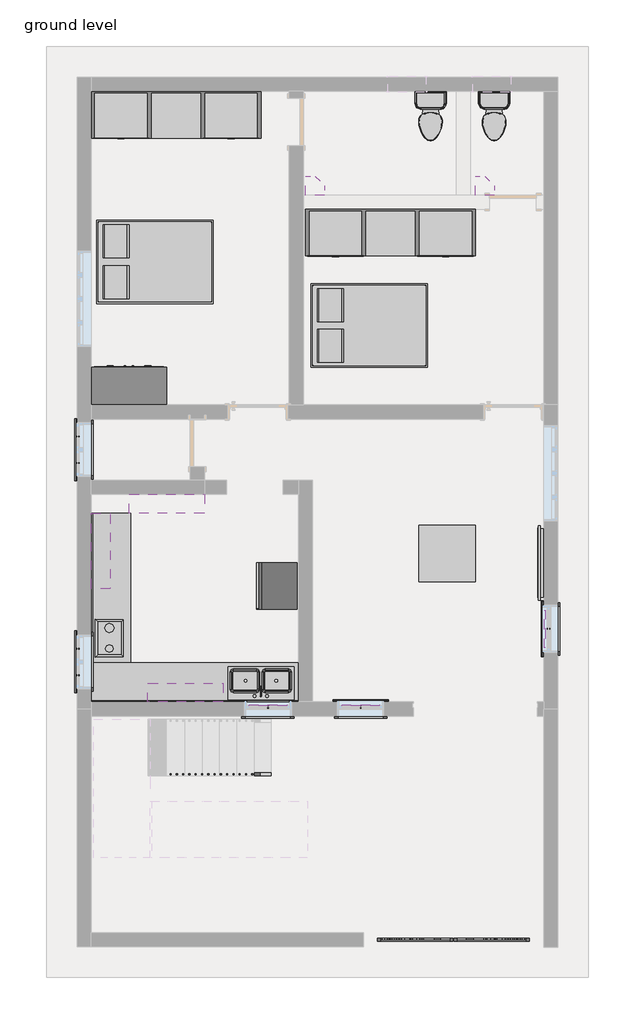
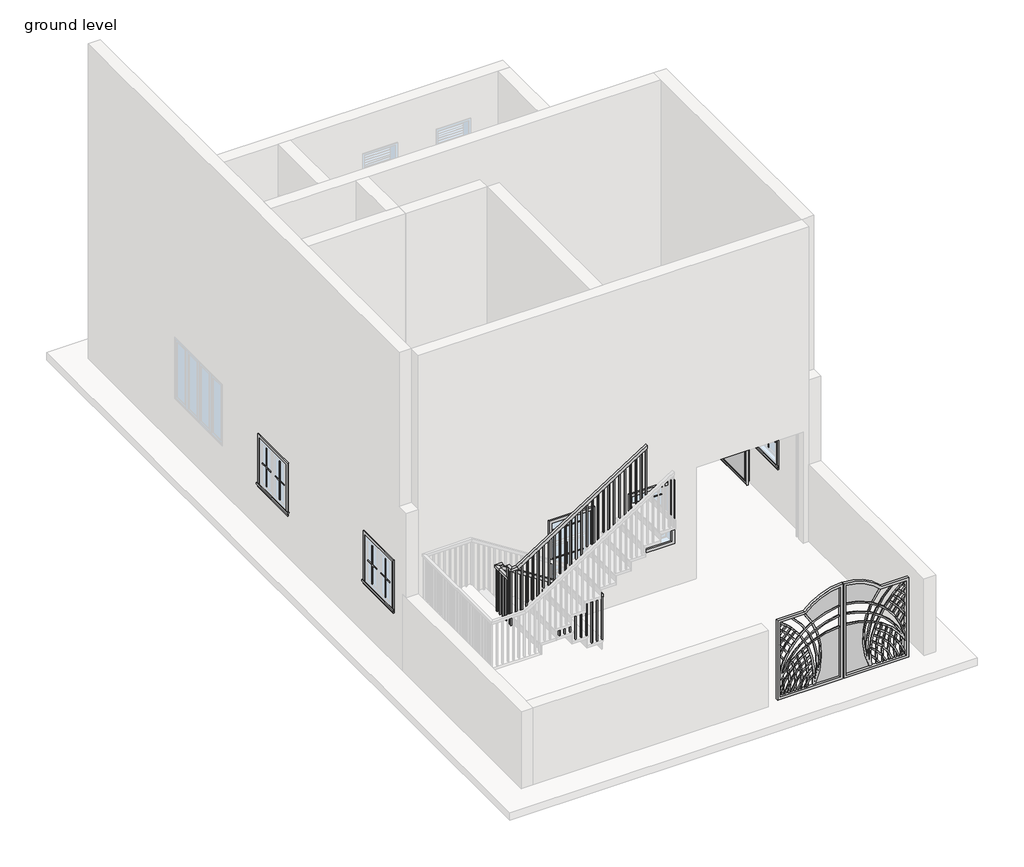
# One storey, part 3 of 3: 23 proxies, 16 furniture elements, 5 flow terminals, 1 railing.
"""IFC4 building model written with IfcOpenShell, lengths in millimetres."""

from ifc_helpers import new_model, si_unit, frame, origin, place, context, project, spatial, polyline, outline, extrude, faceted_brep, transform, mapped, element, save
from components import generic_models_6bc30956, proxy_3c1fa1d0, muntin_pattern_2x2_muntin_pattern_2x2_b3fe6957, muntin_pattern_2x2_muntin_pattern_2x2_3e0ecaf2, muntin_pattern_2x2_muntin_pattern_2x2_b8ba09c9, proxy_76352e5b, trim_window_exterior_flat_with_sill_41619996, trim_window_exterior_flat_with_sill_6cd3ad68, trim_window_interior_flat_picture_frame_51c85655, trim_window_interior_flat_picture_frame_840a62db, flow_terminal_080557f2, flow_terminal_a53be723, toilet_domestic_3d_toilet_domestic_3d_ba6479b0, toilet_domestic_3d_toilet_domestic_3d_30431060, furniture_9b4ba0d7, furniture_3428e43d, furniture_97fe820d, furniture_b58f7881, furniture_05b7e736, furniture_e3ff1115, furniture_1f19b6cd, furniture_8a11f05f, furniture_5e39d705, furniture_f491f192, furniture_82e269c4

model = new_model("IFC4")

# Units and contexts
model_context = context("Model", 3, world=origin())
ifc_project = project(units=[si_unit("LENGTHUNIT", "METRE", prefix="MILLI")], contexts=[model_context])

# Site, building, storey
site = spatial("IfcSite", under=ifc_project)
building = spatial("IfcBuilding", under=site)
storey = spatial("IfcBuildingStorey", under=building, Name="ground level", Elevation=609.6)

# Proxies
placement = place(None, origin())
generic_models_shape = generic_models_6bc30956(model_context)
element("IfcBuildingElementProxy", 1, Name="Generic Models", at=placement, inside=storey, context=model_context, shape_type="MappedRepresentation", body=[
    mapped(generic_models_shape, transform((34462.4566163, 5742.2730552, 609.6), x_axis=(1.0, 0.0, 0.0), y_axis=(0.0, 1.0, 0.0), z_axis=(0.0, 0.0, 1.0))),
])
proxy_shape = proxy_3c1fa1d0(model_context)
element("IfcBuildingElementProxy", 2, Name="Cook Top-2 Unit : 12\" x 18\" 2", ObjectType="Cook Top-2 Unit : 12\" x 18\" 2", at=placement, inside=storey, context=model_context, shape_type="MappedRepresentation", body=[
    mapped(proxy_shape, transform((28826.8316163, 10560.2732596, 609.6), x_axis=(1.0, 0.0, 0.0), y_axis=(0.0, 1.0, 0.0), z_axis=(0.0, 0.0, 1.0))),
])
muntin_pattern_2x2_muntin_pattern_2x2_shape = muntin_pattern_2x2_muntin_pattern_2x2_b3fe6957(model_context)
element("IfcBuildingElementProxy", 3, Name="Muntin Pattern_2x2 : Muntin Pattern_2x2", ObjectType="Muntin Pattern_2x2 : Muntin Pattern_2x2", at=placement, inside=storey, context=model_context, shape_type="MappedRepresentation", body=[
    mapped(muntin_pattern_2x2_muntin_pattern_2x2_shape, transform((28391.8566163, 13424.1855552, 1593.85), x_axis=(0.0, 1.0, 0.0), y_axis=(-1.0, 0.0, 0.0), z_axis=(0.0, 0.0, 1.0))),
])
element("IfcBuildingElementProxy", 4, Name="Muntin Pattern_2x2 : Muntin Pattern_2x2", ObjectType="Muntin Pattern_2x2 : Muntin Pattern_2x2", at=placement, inside=storey, context=model_context, shape_type="MappedRepresentation", body=[
    mapped(muntin_pattern_2x2_muntin_pattern_2x2_shape, transform((28391.8566163, 9995.1855552, 1746.25), x_axis=(0.0, 1.0, 0.0), y_axis=(-1.0, 0.0, 0.0), z_axis=(0.0, 0.0, 1.0))),
])
muntin_pattern_2x2_muntin_pattern_2x2_2_shape = muntin_pattern_2x2_muntin_pattern_2x2_3e0ecaf2(model_context)
element("IfcBuildingElementProxy", 5, Name="Muntin Pattern_2x2 : Muntin Pattern_2x2", ObjectType="Muntin Pattern_2x2 : Muntin Pattern_2x2", at=placement, inside=storey, context=model_context, shape_type="MappedRepresentation", body=[
    mapped(muntin_pattern_2x2_muntin_pattern_2x2_2_shape, transform((28391.8566163, 13852.8105552, 1593.85), x_axis=(0.0, -1.0, 0.0), y_axis=(1.0, 0.0, 0.0), z_axis=(0.0, 0.0, 1.0))),
])
element("IfcBuildingElementProxy", 6, Name="Muntin Pattern_2x2 : Muntin Pattern_2x2", ObjectType="Muntin Pattern_2x2 : Muntin Pattern_2x2", at=placement, inside=storey, context=model_context, shape_type="MappedRepresentation", body=[
    mapped(muntin_pattern_2x2_muntin_pattern_2x2_2_shape, transform((28391.8566163, 10423.8105552, 1746.25), x_axis=(0.0, -1.0, 0.0), y_axis=(1.0, 0.0, 0.0), z_axis=(0.0, 0.0, 1.0))),
])
muntin_pattern_2x2_muntin_pattern_2x2_3_shape = muntin_pattern_2x2_muntin_pattern_2x2_b8ba09c9(model_context)
element("IfcBuildingElementProxy", 7, Name="Muntin Pattern_2x2 : Muntin Pattern_2x2", ObjectType="Muntin Pattern_2x2 : Muntin Pattern_2x2", at=placement, inside=storey, context=model_context, shape_type="MappedRepresentation", body=[
    mapped(muntin_pattern_2x2_muntin_pattern_2x2_3_shape, transform((32967.0316163, 9526.8730552, 2130.425), x_axis=(1.0, 0.0, 0.0), y_axis=(0.0, 1.0, 0.0), z_axis=(0.0, 0.0, 1.0))),
])
element("IfcBuildingElementProxy", 8, Name="Muntin Pattern_2x2 : Muntin Pattern_2x2", ObjectType="Muntin Pattern_2x2 : Muntin Pattern_2x2", at=placement, inside=storey, context=model_context, shape_type="MappedRepresentation", body=[
    mapped(muntin_pattern_2x2_muntin_pattern_2x2_3_shape, transform((32967.0316163, 9482.4230552, 1600.2), x_axis=(1.0, 0.0, 0.0), y_axis=(0.0, 1.0, 0.0), z_axis=(0.0, 0.0, 1.0))),
])
element("IfcBuildingElementProxy", 9, Name="Muntin Pattern_2x2 : Muntin Pattern_2x2", ObjectType="Muntin Pattern_2x2 : Muntin Pattern_2x2", at=placement, inside=storey, context=model_context, shape_type="MappedRepresentation", body=[
    mapped(muntin_pattern_2x2_muntin_pattern_2x2_3_shape, transform((35961.0566163, 10742.8980552, 2130.425), x_axis=(0.0, 1.0, 0.0), y_axis=(-1.0, 0.0, 0.0), z_axis=(0.0, 0.0, 1.0))),
])
element("IfcBuildingElementProxy", 10, Name="Muntin Pattern_2x2 : Muntin Pattern_2x2", ObjectType="Muntin Pattern_2x2 : Muntin Pattern_2x2", at=placement, inside=storey, context=model_context, shape_type="MappedRepresentation", body=[
    mapped(muntin_pattern_2x2_muntin_pattern_2x2_3_shape, transform((36005.5066163, 10742.8980552, 1600.2), x_axis=(0.0, 1.0, 0.0), y_axis=(-1.0, 0.0, 0.0), z_axis=(0.0, 0.0, 1.0))),
])
element("IfcBuildingElementProxy", 11, Name="Muntin Pattern_2x2 : Muntin Pattern_2x2", ObjectType="Muntin Pattern_2x2 : Muntin Pattern_2x2", at=placement, inside=storey, context=model_context, shape_type="MappedRepresentation", body=[
    mapped(muntin_pattern_2x2_muntin_pattern_2x2_3_shape, transform((31468.4316163, 9526.8730552, 2130.425), x_axis=(1.0, 0.0, 0.0), y_axis=(0.0, 1.0, 0.0), z_axis=(0.0, 0.0, 1.0))),
])
element("IfcBuildingElementProxy", 12, Name="Muntin Pattern_2x2 : Muntin Pattern_2x2", ObjectType="Muntin Pattern_2x2 : Muntin Pattern_2x2", at=placement, inside=storey, context=model_context, shape_type="MappedRepresentation", body=[
    mapped(muntin_pattern_2x2_muntin_pattern_2x2_3_shape, transform((31468.4316163, 9482.4230552, 1600.2), x_axis=(1.0, 0.0, 0.0), y_axis=(0.0, 1.0, 0.0), z_axis=(0.0, 0.0, 1.0))),
])
proxy_2_shape = proxy_76352e5b(model_context)
element("IfcBuildingElementProxy", 13, Name="Refrigerator-Built-in : 30\" x 24\" LH", ObjectType="Refrigerator-Built-in : 30\" x 24\" LH", at=placement, inside=storey, context=model_context, shape_type="MappedRepresentation", body=[
    mapped(proxy_2_shape, transform((31644.2555878, 11435.0480552, 609.6), x_axis=(0.0, 1.0, 0.0), y_axis=(-1.0, 0.0, 0.0), z_axis=(0.0, 0.0, 1.0))),
])
trim_window_exterior_flat_with_sill_shape = trim_window_exterior_flat_with_sill_41619996(model_context)
element("IfcBuildingElementProxy", 14, Name="Trim-Window-Exterior-Flat : with Sill", ObjectType="Trim-Window-Exterior-Flat : with Sill", at=placement, inside=storey, context=model_context, shape_type="MappedRepresentation", body=[
    mapped(trim_window_exterior_flat_with_sill_shape, transform((28382.3316163, 13638.4980552, 2438.4), x_axis=(0.0, -1.0, 0.0), y_axis=(0.0, 0.0, 1.0), z_axis=(-1.0, 0.0, 0.0))),
])
element("IfcBuildingElementProxy", 15, Name="Trim-Window-Exterior-Flat : with Sill", ObjectType="Trim-Window-Exterior-Flat : with Sill", at=placement, inside=storey, context=model_context, shape_type="MappedRepresentation", body=[
    mapped(trim_window_exterior_flat_with_sill_shape, transform((28382.3316163, 10209.4980552, 2590.8), x_axis=(0.0, -1.0, 0.0), y_axis=(0.0, 0.0, 1.0), z_axis=(-1.0, 0.0, 0.0))),
])
trim_window_exterior_flat_with_sill_2_shape = trim_window_exterior_flat_with_sill_6cd3ad68(model_context)
element("IfcBuildingElementProxy", 16, Name="Trim-Window-Exterior-Flat : with Sill", ObjectType="Trim-Window-Exterior-Flat : with Sill", at=placement, inside=storey, context=model_context, shape_type="MappedRepresentation", body=[
    mapped(trim_window_exterior_flat_with_sill_2_shape, transform((32967.0316163, 9561.7980552, 2692.4), x_axis=(-1.0, 0.0, 0.0), y_axis=(0.0, 0.0, 1.0), z_axis=(0.0, 1.0, 0.0))),
])
element("IfcBuildingElementProxy", 17, Name="Trim-Window-Exterior-Flat : with Sill", ObjectType="Trim-Window-Exterior-Flat : with Sill", at=placement, inside=storey, context=model_context, shape_type="MappedRepresentation", body=[
    mapped(trim_window_exterior_flat_with_sill_2_shape, transform((35926.1316163, 10742.8980552, 2692.4), x_axis=(0.0, -1.0, 0.0), y_axis=(0.0, 0.0, 1.0), z_axis=(-1.0, 0.0, 0.0))),
])
element("IfcBuildingElementProxy", 18, Name="Trim-Window-Exterior-Flat : with Sill", ObjectType="Trim-Window-Exterior-Flat : with Sill", at=placement, inside=storey, context=model_context, shape_type="MappedRepresentation", body=[
    mapped(trim_window_exterior_flat_with_sill_2_shape, transform((31468.4316163, 9561.7980552, 2692.4), x_axis=(-1.0, 0.0, 0.0), y_axis=(0.0, 0.0, 1.0), z_axis=(0.0, 1.0, 0.0))),
])
trim_window_interior_flat_picture_frame_shape = trim_window_interior_flat_picture_frame_51c85655(model_context)
element("IfcBuildingElementProxy", 19, Name="Trim-Window-Interior-Flat : Picture Frame", ObjectType="Trim-Window-Interior-Flat : Picture Frame", at=placement, inside=storey, context=model_context, shape_type="MappedRepresentation", body=[
    mapped(trim_window_interior_flat_picture_frame_shape, transform((28610.9316163, 13638.4980552, 2438.4), x_axis=(0.0, 1.0, 0.0), y_axis=(0.0, 0.0, 1.0), z_axis=(1.0, 0.0, 0.0))),
])
element("IfcBuildingElementProxy", 20, Name="Trim-Window-Interior-Flat : Picture Frame", ObjectType="Trim-Window-Interior-Flat : Picture Frame", at=placement, inside=storey, context=model_context, shape_type="MappedRepresentation", body=[
    mapped(trim_window_interior_flat_picture_frame_shape, transform((28610.9316163, 10209.4980552, 2590.8), x_axis=(0.0, 1.0, 0.0), y_axis=(0.0, 0.0, 1.0), z_axis=(1.0, 0.0, 0.0))),
])
trim_window_interior_flat_picture_frame_2_shape = trim_window_interior_flat_picture_frame_840a62db(model_context)
element("IfcBuildingElementProxy", 21, Name="Trim-Window-Interior-Flat : Picture Frame", ObjectType="Trim-Window-Interior-Flat : Picture Frame", at=placement, inside=storey, context=model_context, shape_type="MappedRepresentation", body=[
    mapped(trim_window_interior_flat_picture_frame_2_shape, transform((32967.0316163, 9333.1980552, 2692.4), x_axis=(1.0, 0.0, 0.0), y_axis=(0.0, 0.0, 1.0), z_axis=(0.0, -1.0, 0.0))),
])
element("IfcBuildingElementProxy", 22, Name="Trim-Window-Interior-Flat : Picture Frame", ObjectType="Trim-Window-Interior-Flat : Picture Frame", at=placement, inside=storey, context=model_context, shape_type="MappedRepresentation", body=[
    mapped(trim_window_interior_flat_picture_frame_2_shape, transform((36154.7316163, 10742.8980552, 2692.4), x_axis=(0.0, 1.0, 0.0), y_axis=(0.0, 0.0, 1.0), z_axis=(1.0, 0.0, 0.0))),
])
element("IfcBuildingElementProxy", 23, Name="Trim-Window-Interior-Flat : Picture Frame", ObjectType="Trim-Window-Interior-Flat : Picture Frame", at=placement, inside=storey, context=model_context, shape_type="MappedRepresentation", body=[
    mapped(trim_window_interior_flat_picture_frame_2_shape, transform((31468.4316163, 9333.1980552, 2692.4), x_axis=(1.0, 0.0, 0.0), y_axis=(0.0, 0.0, 1.0), z_axis=(0.0, -1.0, 0.0))),
])

# Flow terminals
flow_terminal_shape = flow_terminal_080557f2(model_context)
element("IfcFlowTerminal", 24, ObjectType="Sink - Mop : 28\"x28\" 2", at=placement, inside=storey, context=model_context, shape_type="MappedRepresentation", body=[
    mapped(flow_terminal_shape, transform((32078.0316163, 17753.2980552, 1828.8), x_axis=(0.0, 1.0, 0.0), y_axis=(-1.0, 0.0, 0.0), z_axis=(0.0, 0.0, 1.0))),
])
element("IfcFlowTerminal", 25, ObjectType="Sink - Mop : 28\"x28\" 2", at=placement, inside=storey, context=model_context, shape_type="MappedRepresentation", body=[
    mapped(flow_terminal_shape, transform((34821.2316163, 17753.2980552, 1828.8), x_axis=(0.0, 1.0, 0.0), y_axis=(-1.0, 0.0, 0.0), z_axis=(0.0, 0.0, 1.0))),
])
flow_terminal_2_shape = flow_terminal_a53be723(model_context)
element("IfcFlowTerminal", 26, ObjectType="Sink Kitchen-Double : 42\" x 21\"", at=placement, inside=storey, context=model_context, shape_type="MappedRepresentation", body=[
    mapped(flow_terminal_2_shape, transform((31369.8208569, 9868.9434563, 609.6), x_axis=(-1.0, 0.0, 0.0), y_axis=(0.0, -1.0, 0.0), z_axis=(0.0, 0.0, 1.0))),
])
toilet_domestic_3d_toilet_domestic_3d_shape = toilet_domestic_3d_toilet_domestic_3d_ba6479b0(model_context)
toilet_domestic_3d_toilet_domestic_3d_2_shape = toilet_domestic_3d_toilet_domestic_3d_30431060(model_context)
element("IfcFlowTerminal", 27, ObjectType="Toilet-Domestic-3D : Toilet-Domestic-3D", at=placement, inside=storey, context=model_context, shape_type="MappedRepresentation", body=[
    mapped(toilet_domestic_3d_toilet_domestic_3d_shape, transform((34097.3316163, 18935.0020278, 609.6), x_axis=(1.0, 0.0, 0.0), y_axis=(0.0, 1.0, 0.0), z_axis=(0.0, 0.0, 1.0))),
    mapped(toilet_domestic_3d_toilet_domestic_3d_2_shape, transform((34097.3316163, 18935.0020278, 609.6), x_axis=(1.0, 0.0, 0.0), y_axis=(0.0, 1.0, 0.0), z_axis=(0.0, 0.0, 1.0))),
])
element("IfcFlowTerminal", 28, ObjectType="Toilet-Domestic-3D : Toilet-Domestic-3D", at=placement, inside=storey, context=model_context, shape_type="MappedRepresentation", body=[
    mapped(toilet_domestic_3d_toilet_domestic_3d_shape, transform((35126.0316163, 18935.0020278, 609.6), x_axis=(1.0, 0.0, 0.0), y_axis=(0.0, 1.0, 0.0), z_axis=(0.0, 0.0, 1.0))),
    mapped(toilet_domestic_3d_toilet_domestic_3d_2_shape, transform((35126.0316163, 18935.0020278, 609.6), x_axis=(1.0, 0.0, 0.0), y_axis=(0.0, 1.0, 0.0), z_axis=(0.0, 0.0, 1.0))),
])

# Furniture
furniture_shape = furniture_9b4ba0d7(model_context)
element("IfcFurniture", 29, ObjectType="36\"", at=placement, inside=storey, context=model_context, shape_type="MappedRepresentation", body=[
    mapped(furniture_shape, transform((28610.9316163, 12133.8603503, 609.6), x_axis=(0.0, 1.0, 0.0), y_axis=(-1.0, 0.0, 0.0), z_axis=(0.0, 0.0, 1.0))),
])
furniture_2_shape = furniture_3428e43d(model_context)
element("IfcFurniture", 30, ObjectType="48\"", at=placement, inside=storey, context=model_context, shape_type="MappedRepresentation", body=[
    mapped(furniture_2_shape, transform((30225.7765763, 9561.7980552, 609.6), x_axis=(-1.0, 0.0, 0.0), y_axis=(0.0, -1.0, 0.0), z_axis=(0.0, 0.0, 1.0))),
])
element("IfcFurniture", 31, ObjectType="48\"", at=placement, inside=storey, context=model_context, shape_type="MappedRepresentation", body=[
    mapped(furniture_2_shape, transform((28610.9316163, 10994.9530952, 609.6), x_axis=(0.0, 1.0, 0.0), y_axis=(-1.0, 0.0, 0.0), z_axis=(0.0, 0.0, 1.0))),
])
furniture_3_shape = furniture_97fe820d(model_context)
element("IfcFurniture", 32, ObjectType="Base Cabinet-Corner Unit-Square : 36\"", at=placement, inside=storey, context=model_context, shape_type="MappedRepresentation", body=[
    mapped(furniture_3_shape, transform((29137.6693213, 9561.7980552, 609.6), x_axis=(-1.0, 0.0, 0.0), y_axis=(0.0, -1.0, 0.0), z_axis=(0.0, 0.0, 1.0))),
])
furniture_4_shape = furniture_b58f7881(model_context)
element("IfcFurniture", 33, ObjectType="Bed-Box : Double 53\" x 74\"", at=placement, inside=storey, context=model_context, shape_type="MappedRepresentation", body=[
    mapped(furniture_4_shape, transform((29405.2021081, 16334.6455962, 609.6), x_axis=(0.0, 1.0, 0.0), y_axis=(-1.0, 0.0, 0.0), z_axis=(0.0, 0.0, 1.0))),
])
element("IfcFurniture", 34, ObjectType="Bed-Box : Double 53\" x 74\"", at=placement, inside=storey, context=model_context, shape_type="MappedRepresentation", body=[
    mapped(furniture_4_shape, transform((32872.3021081, 15305.9455962, 609.6), x_axis=(0.0, 1.0, 0.0), y_axis=(-1.0, 0.0, 0.0), z_axis=(0.0, 0.0, 1.0))),
])
furniture_5_shape = furniture_05b7e736(model_context)
element("IfcFurniture", 35, ObjectType="Counter Top : 24\" Depth", at=placement, inside=storey, context=model_context, shape_type="MappedRepresentation", body=[
    mapped(furniture_5_shape, transform((28610.9316163, 11397.2603503, 609.6), x_axis=(0.0, 1.0, 0.0), y_axis=(-1.0, 0.0, 0.0), z_axis=(0.0, 0.0, 1.0))),
])
furniture_6_shape = furniture_e3ff1115(model_context)
element("IfcFurniture", 36, ObjectType="Counter Top w Sink : 24\" Depth", at=placement, inside=storey, context=model_context, shape_type="MappedRepresentation", body=[
    mapped(furniture_6_shape, transform((30763.2693213, 9561.7980552, 609.6), x_axis=(-1.0, 0.0, 0.0), y_axis=(0.0, -1.0, 0.0), z_axis=(0.0, 0.0, 1.0))),
])
furniture_7_shape = furniture_1f19b6cd(model_context)
element("IfcFurniture", 37, ObjectType="Entertainment Center.0001 : 96\" x 84\" x 30\"", at=placement, inside=storey, context=model_context, shape_type="MappedRepresentation", body=[
    mapped(furniture_7_shape, transform((29982.5316163, 19455.0980552, 609.6), x_axis=(1.0, 0.0, 0.0), y_axis=(0.0, 1.0, 0.0), z_axis=(0.0, 0.0, 1.0))),
])
element("IfcFurniture", 38, ObjectType="Entertainment Center.0001 : 96\" x 84\" x 30\"", at=placement, inside=storey, context=model_context, shape_type="MappedRepresentation", body=[
    mapped(furniture_7_shape, transform((33449.6316163, 17550.0980552, 609.6), x_axis=(1.0, 0.0, 0.0), y_axis=(0.0, 1.0, 0.0), z_axis=(0.0, 0.0, 1.0))),
])
furniture_8_shape = furniture_8a11f05f(model_context)
element("IfcFurniture", 39, ObjectType="Table-Rectangular : 36\" x 36\" 2", at=placement, inside=storey, context=model_context, shape_type="MappedRepresentation", body=[
    mapped(furniture_8_shape, transform((34364.0316163, 11962.0980552, 609.6), x_axis=(1.0, 0.0, 0.0), y_axis=(0.0, 1.0, 0.0), z_axis=(0.0, 0.0, 1.0))),
])
furniture_9_shape = furniture_5e39d705(model_context)
element("IfcFurniture", 40, ObjectType="Television-Plasma : 50\"", at=placement, inside=storey, context=model_context, shape_type="MappedRepresentation", body=[
    mapped(furniture_9_shape, transform((35926.1316163, 11866.8480552, 609.6), x_axis=(0.0, -1.0, 0.0), y_axis=(1.0, 0.0, 0.0), z_axis=(0.0, 0.0, 1.0))),
])
furniture_10_shape = furniture_f491f192(model_context)
element("IfcFurniture", 41, ObjectType="Upper Cabinet-Pass-Thru w Glass : 48\" x 30\" x 12\"", at=placement, inside=storey, context=model_context, shape_type="MappedRepresentation", body=[
    mapped(furniture_10_shape, transform((28610.9316163, 11981.4603503, 609.6), x_axis=(0.0, 1.0, 0.0), y_axis=(-1.0, 0.0, 0.0), z_axis=(0.0, 0.0, 1.0))),
])
element("IfcFurniture", 42, ObjectType="Upper Cabinet-Pass-Thru w Glass : 48\" x 30\" x 12\"", at=placement, inside=storey, context=model_context, shape_type="MappedRepresentation", body=[
    mapped(furniture_10_shape, transform((29848.8693213, 12609.7980552, 609.6), x_axis=(-1.0, 0.0, 0.0), y_axis=(0.0, -1.0, 0.0), z_axis=(0.0, 0.0, 1.0))),
])
element("IfcFurniture", 43, ObjectType="Upper Cabinet-Pass-Thru w Glass : 48\" x 30\" x 12\"", at=placement, inside=storey, context=model_context, shape_type="MappedRepresentation", body=[
    mapped(furniture_10_shape, transform((30153.6693213, 9561.7980552, 609.6), x_axis=(-1.0, 0.0, 0.0), y_axis=(0.0, -1.0, 0.0), z_axis=(0.0, 0.0, 1.0))),
])
furniture_11_shape = furniture_82e269c4(model_context)
element("IfcFurniture", 44, ObjectType="Wardrobe : 48\" x 72\" x 24\"", at=placement, inside=storey, context=model_context, shape_type="MappedRepresentation", body=[
    mapped(furniture_11_shape, transform((28951.3383565, 14083.4592456, 609.6), x_axis=(-1.0, 0.0, 0.0), y_axis=(0.0, -1.0, 0.0), z_axis=(0.0, 0.0, 1.0))),
])

# Railing
element("IfcRailing", 45, ObjectType="Handrail - Rectangular", at=placement, inside=storey, context=model_context, shape_type="SolidModel", body=[
    faceted_brep([(31519.2316163, 8367.9980552, 1701.8), (31519.2316163, 8367.9980552, 1641.586276), (31519.2316163, 8418.7980552, 1641.586276), (31519.2316163, 8418.7980552, 1701.8), (29639.6316163, 8367.9980552, 2897.9090909), (29588.8316163, 8367.9980552, 2870.0226396), (29588.8316163, 8418.7980552, 2870.0226396), (29639.6316163, 8418.7980552, 2897.9090909), (29639.6316163, 8367.9980552, 2946.4), (29588.8316163, 8367.9980552, 2895.6), (29588.8316163, 8418.7980552, 2895.6), (29639.6316163, 8418.7980552, 2946.4), (29563.4316163, 8367.9980552, 2946.4), (29563.4316163, 8367.9980552, 2895.6), (29512.6316163, 8418.7980552, 2895.6), (29512.6316163, 8418.7980552, 2946.4), (29563.4316163, 8291.7980552, 2946.4), (29563.4316163, 8291.7980552, 2895.6), (29512.6316163, 8291.7980552, 2895.6), (29512.6316163, 8291.7980552, 2946.4), (29563.4316163, 8031.4480552, 2946.4), (29563.4316163, 7980.6480552, 2895.6), (29512.6316163, 7980.6480552, 2895.6), (29512.6316163, 8031.4480552, 2946.4), (29563.4316163, 8031.4480552, 3172.6909091), (29563.4316163, 7980.6480552, 3121.8909091), (29512.6316163, 7980.6480552, 3121.8909091), (29512.6316163, 8031.4480552, 3172.6909091), (29563.4316163, 7955.2480552, 3172.6909091), (29563.4316163, 7955.2480552, 3121.8909091), (29512.6316163, 7904.4480552, 3121.8909091), (29512.6316163, 7904.4480552, 3172.6909091), (29639.6316163, 7955.2480552, 3172.6909091), (29654.4246113, 7955.2480552, 3121.8909091), (29654.4246113, 7904.4480552, 3121.8909091), (29639.6316163, 7904.4480552, 3172.6909091), (32078.0316163, 7955.2480552, 4724.4), (32078.0316163, 7904.4480552, 4724.4), (32078.0316163, 7904.4480552, 4664.186276), (32078.0316163, 7955.2480552, 4664.186276)], [[[0, 1, 2, 3]], [[1, 0, 4, 5]], [[2, 1, 5, 6]], [[3, 2, 6, 7]], [[0, 3, 7, 4]], [[5, 4, 8, 9]], [[6, 5, 9, 10]], [[7, 6, 10, 11]], [[4, 7, 11, 8]], [[9, 8, 12, 13]], [[10, 9, 13, 14]], [[11, 10, 14, 15]], [[8, 11, 15, 12]], [[13, 12, 16, 17]], [[14, 13, 17, 18]], [[15, 14, 18, 19]], [[12, 15, 19, 16]], [[17, 16, 20, 21]], [[18, 17, 21, 22]], [[19, 18, 22, 23]], [[16, 19, 23, 20]], [[21, 20, 24, 25]], [[22, 21, 25, 26]], [[23, 22, 26, 27]], [[20, 23, 27, 24]], [[25, 24, 28, 29]], [[26, 25, 29, 30]], [[27, 26, 30, 31]], [[24, 27, 31, 28]], [[29, 28, 32, 33]], [[30, 29, 33, 34]], [[31, 30, 34, 35]], [[28, 31, 35, 32]], [[36, 37, 38, 39]], [[33, 32, 36, 39]], [[34, 33, 39, 38]], [[35, 34, 38, 37]], [[32, 35, 37, 36]]]),
    extrude(outline(polyline([(4593.4703669, 31966.9066163), (3632.2, 31966.9066163), (3632.2, 31985.9566163), (4605.5930941, 31985.9566163), (4593.4703669, 31966.9066163)])), frame((0.0, 7920.3230552, 0.0), z_axis=(0.0, 1.0, 0.0), x_axis=(0.0, 0.0, 1.0)), (0.0, 0.0, 1.0), 19.05),
    extrude(outline(polyline([(4528.8158214, 31865.3066163), (3632.2, 31865.3066163), (3632.2, 31884.3566163), (4540.9385487, 31884.3566163), (4528.8158214, 31865.3066163)])), frame((0.0, 7920.3230552, 0.0), z_axis=(0.0, 1.0, 0.0), x_axis=(0.0, 0.0, 1.0)), (0.0, 0.0, 1.0), 19.05),
    extrude(outline(polyline([(4464.161276, 31763.7066163), (3454.4, 31763.7066163), (3454.4, 31782.7566163), (4476.2840032, 31782.7566163), (4464.161276, 31763.7066163)])), frame((0.0, 7920.3230552, 0.0), z_axis=(0.0, 1.0, 0.0), x_axis=(0.0, 0.0, 1.0)), (0.0, 0.0, 1.0), 19.05),
    extrude(outline(polyline([(4399.5067305, 31662.1066163), (3454.4, 31662.1066163), (3454.4, 31681.1566163), (4411.6294578, 31681.1566163), (4399.5067305, 31662.1066163)])), frame((0.0, 7920.3230552, 0.0), z_axis=(0.0, 1.0, 0.0), x_axis=(0.0, 0.0, 1.0)), (0.0, 0.0, 1.0), 19.05),
    extrude(outline(polyline([(4334.8521851, 31560.5066163), (3454.4, 31560.5066163), (3454.4, 31579.5566163), (4346.9749123, 31579.5566163), (4334.8521851, 31560.5066163)])), frame((0.0, 7920.3230552, 0.0), z_axis=(0.0, 1.0, 0.0), x_axis=(0.0, 0.0, 1.0)), (0.0, 0.0, 1.0), 19.05),
    extrude(outline(polyline([(4270.1976396, 31458.9066163), (3276.6, 31458.9066163), (3276.6, 31477.9566163), (4282.3203669, 31477.9566163), (4270.1976396, 31458.9066163)])), frame((0.0, 7920.3230552, 0.0), z_axis=(0.0, 1.0, 0.0), x_axis=(0.0, 0.0, 1.0)), (0.0, 0.0, 1.0), 19.05),
    extrude(outline(polyline([(4205.5430941, 31357.3066163), (3276.6, 31357.3066163), (3276.6, 31376.3566163), (4217.6658214, 31376.3566163), (4205.5430941, 31357.3066163)])), frame((0.0, 7920.3230552, 0.0), z_axis=(0.0, 1.0, 0.0), x_axis=(0.0, 0.0, 1.0)), (0.0, 0.0, 1.0), 19.05),
    extrude(outline(polyline([(4140.8885487, 31255.7066163), (3276.6, 31255.7066163), (3276.6, 31274.7566163), (4153.011276, 31274.7566163), (4140.8885487, 31255.7066163)])), frame((0.0, 7920.3230552, 0.0), z_axis=(0.0, 1.0, 0.0), x_axis=(0.0, 0.0, 1.0)), (0.0, 0.0, 1.0), 19.05),
    extrude(outline(polyline([(4076.2340032, 31154.1066163), (3098.8, 31154.1066163), (3098.8, 31173.1566163), (4088.3567305, 31173.1566163), (4076.2340032, 31154.1066163)])), frame((0.0, 7920.3230552, 0.0), z_axis=(0.0, 1.0, 0.0), x_axis=(0.0, 0.0, 1.0)), (0.0, 0.0, 1.0), 19.05),
    extrude(outline(polyline([(4011.5794578, 31052.5066163), (3098.8, 31052.5066163), (3098.8, 31071.5566163), (4023.7021851, 31071.5566163), (4011.5794578, 31052.5066163)])), frame((0.0, 7920.3230552, 0.0), z_axis=(0.0, 1.0, 0.0), x_axis=(0.0, 0.0, 1.0)), (0.0, 0.0, 1.0), 19.05),
    extrude(outline(polyline([(3946.9249123, 30950.9066163), (3098.8, 30950.9066163), (3098.8, 30969.9566163), (3959.0476396, 30969.9566163), (3946.9249123, 30950.9066163)])), frame((0.0, 7920.3230552, 0.0), z_axis=(0.0, 1.0, 0.0), x_axis=(0.0, 0.0, 1.0)), (0.0, 0.0, 1.0), 19.05),
    extrude(outline(polyline([(3882.2703669, 30849.3066163), (2921.0, 30849.3066163), (2921.0, 30868.3566163), (3894.3930941, 30868.3566163), (3882.2703669, 30849.3066163)])), frame((0.0, 7920.3230552, 0.0), z_axis=(0.0, 1.0, 0.0), x_axis=(0.0, 0.0, 1.0)), (0.0, 0.0, 1.0), 19.05),
    extrude(outline(polyline([(3817.6158214, 30747.7066163), (2921.0, 30747.7066163), (2921.0, 30766.7566163), (3829.7385487, 30766.7566163), (3817.6158214, 30747.7066163)])), frame((0.0, 7920.3230552, 0.0), z_axis=(0.0, 1.0, 0.0), x_axis=(0.0, 0.0, 1.0)), (0.0, 0.0, 1.0), 19.05),
    extrude(outline(polyline([(3752.961276, 30646.1066163), (2743.2, 30646.1066163), (2743.2, 30665.1566163), (3765.0840032, 30665.1566163), (3752.961276, 30646.1066163)])), frame((0.0, 7920.3230552, 0.0), z_axis=(0.0, 1.0, 0.0), x_axis=(0.0, 0.0, 1.0)), (0.0, 0.0, 1.0), 19.05),
    extrude(outline(polyline([(3688.3067305, 30544.5066163), (2743.2, 30544.5066163), (2743.2, 30563.5566163), (3700.4294578, 30563.5566163), (3688.3067305, 30544.5066163)])), frame((0.0, 7920.3230552, 0.0), z_axis=(0.0, 1.0, 0.0), x_axis=(0.0, 0.0, 1.0)), (0.0, 0.0, 1.0), 19.05),
    extrude(outline(polyline([(3623.6521851, 30442.9066163), (2743.2, 30442.9066163), (2743.2, 30461.9566163), (3635.7749123, 30461.9566163), (3623.6521851, 30442.9066163)])), frame((0.0, 7920.3230552, 0.0), z_axis=(0.0, 1.0, 0.0), x_axis=(0.0, 0.0, 1.0)), (0.0, 0.0, 1.0), 19.05),
    extrude(outline(polyline([(3558.9976396, 30341.3066163), (2565.4, 30341.3066163), (2565.4, 30360.3566163), (3571.1203669, 30360.3566163), (3558.9976396, 30341.3066163)])), frame((0.0, 7920.3230552, 0.0), z_axis=(0.0, 1.0, 0.0), x_axis=(0.0, 0.0, 1.0)), (0.0, 0.0, 1.0), 19.05),
    extrude(outline(polyline([(3494.3430941, 30239.7066163), (2565.4, 30239.7066163), (2565.4, 30258.7566163), (3506.4658214, 30258.7566163), (3494.3430941, 30239.7066163)])), frame((0.0, 7920.3230552, 0.0), z_axis=(0.0, 1.0, 0.0), x_axis=(0.0, 0.0, 1.0)), (0.0, 0.0, 1.0), 19.05),
    extrude(outline(polyline([(3429.6885487, 30138.1066163), (2565.4, 30138.1066163), (2565.4, 30157.1566163), (3441.811276, 30157.1566163), (3429.6885487, 30138.1066163)])), frame((0.0, 7920.3230552, 0.0), z_axis=(0.0, 1.0, 0.0), x_axis=(0.0, 0.0, 1.0)), (0.0, 0.0, 1.0), 19.05),
    extrude(outline(polyline([(3365.0340032, 30036.5066163), (2387.6, 30036.5066163), (2387.6, 30055.5566163), (3377.1567305, 30055.5566163), (3365.0340032, 30036.5066163)])), frame((0.0, 7920.3230552, 0.0), z_axis=(0.0, 1.0, 0.0), x_axis=(0.0, 0.0, 1.0)), (0.0, 0.0, 1.0), 19.05),
    extrude(outline(polyline([(3300.3794578, 29934.9066163), (2387.6, 29934.9066163), (2387.6, 29953.9566163), (3312.5021851, 29953.9566163), (3300.3794578, 29934.9066163)])), frame((0.0, 7920.3230552, 0.0), z_axis=(0.0, 1.0, 0.0), x_axis=(0.0, 0.0, 1.0)), (0.0, 0.0, 1.0), 19.05),
    extrude(outline(polyline([(3235.7249123, 29833.3066163), (2387.6, 29833.3066163), (2387.6, 29852.3566163), (3247.8476396, 29852.3566163), (3235.7249123, 29833.3066163)])), frame((0.0, 7920.3230552, 0.0), z_axis=(0.0, 1.0, 0.0), x_axis=(0.0, 0.0, 1.0)), (0.0, 0.0, 1.0), 19.05),
    extrude(outline(polyline([(3171.0703669, 29731.7066163), (2209.8, 29731.7066163), (2209.8, 29750.7566163), (3183.1930941, 29750.7566163), (3171.0703669, 29731.7066163)])), frame((0.0, 7920.3230552, 0.0), z_axis=(0.0, 1.0, 0.0), x_axis=(0.0, 0.0, 1.0)), (0.0, 0.0, 1.0), 19.05),
    extrude(outline(polyline([(3106.4158214, 29630.1066163), (2209.8, 29630.1066163), (2209.8, 29649.1566163), (3118.5385487, 29649.1566163), (3106.4158214, 29630.1066163)])), frame((0.0, 7920.3230552, 0.0), z_axis=(0.0, 1.0, 0.0), x_axis=(0.0, 0.0, 1.0)), (0.0, 0.0, 1.0), 19.05),
    extrude(outline(polyline([(29547.5566163, 7996.5230552), (29547.5566163, 7977.4730552), (29528.5066163, 7977.4730552), (29528.5066163, 7996.5230552), (29547.5566163, 7996.5230552)])), frame((0.0, 0.0, 2032.0), z_axis=(0.0, 0.0, 1.0), x_axis=(1.0, 0.0, 0.0)), (0.0, 0.0, 1.0), 1089.8909091),
    extrude(outline(polyline([(29547.5566163, 8098.1230552), (29547.5566163, 8079.0730552), (29528.5066163, 8079.0730552), (29528.5066163, 8098.1230552), (29547.5566163, 8098.1230552)])), frame((0.0, 0.0, 2032.0), z_axis=(0.0, 0.0, 1.0), x_axis=(1.0, 0.0, 0.0)), (0.0, 0.0, 1.0), 863.6),
    extrude(outline(polyline([(29547.5566163, 8199.7230552), (29547.5566163, 8180.6730552), (29528.5066163, 8180.6730552), (29528.5066163, 8199.7230552), (29547.5566163, 8199.7230552)])), frame((0.0, 0.0, 2032.0), z_axis=(0.0, 0.0, 1.0), x_axis=(1.0, 0.0, 0.0)), (0.0, 0.0, 1.0), 863.6),
    extrude(outline(polyline([(29547.5566163, 8301.3230552), (29547.5566163, 8282.2730552), (29528.5066163, 8282.2730552), (29528.5066163, 8301.3230552), (29547.5566163, 8301.3230552)])), frame((0.0, 0.0, 2032.0), z_axis=(0.0, 0.0, 1.0), x_axis=(1.0, 0.0, 0.0)), (0.0, 0.0, 1.0), 863.6),
    extrude(outline(polyline([(29598.3566163, 8383.8730552), (29579.3066163, 8383.8730552), (29579.3066163, 8402.9230552), (29598.3566163, 8402.9230552), (29598.3566163, 8383.8730552)])), frame((0.0, 0.0, 1854.2), z_axis=(0.0, 0.0, 1.0), x_axis=(1.0, 0.0, 0.0)), (0.0, 0.0, 1.0), 1041.4),
    extrude(outline(polyline([(2811.4294578, 29680.9066163), (1854.2, 29680.9066163), (1854.2, 29699.9566163), (2799.3067305, 29699.9566163), (2811.4294578, 29680.9066163)])), frame((0.0, 8383.8730552, 0.0), z_axis=(0.0, 1.0, 0.0), x_axis=(0.0, 0.0, 1.0)), (0.0, 0.0, 1.0), 19.05),
    extrude(outline(polyline([(2746.7749123, 29782.5066163), (1854.2, 29782.5066163), (1854.2, 29801.5566163), (2734.6521851, 29801.5566163), (2746.7749123, 29782.5066163)])), frame((0.0, 8383.8730552, 0.0), z_axis=(0.0, 1.0, 0.0), x_axis=(0.0, 0.0, 1.0)), (0.0, 0.0, 1.0), 19.05),
    extrude(outline(polyline([(2682.1203669, 29884.1066163), (1676.4, 29884.1066163), (1676.4, 29903.1566163), (2669.9976396, 29903.1566163), (2682.1203669, 29884.1066163)])), frame((0.0, 8383.8730552, 0.0), z_axis=(0.0, 1.0, 0.0), x_axis=(0.0, 0.0, 1.0)), (0.0, 0.0, 1.0), 19.05),
    extrude(outline(polyline([(2617.4658214, 29985.7066163), (1676.4, 29985.7066163), (1676.4, 30004.7566163), (2605.3430941, 30004.7566163), (2617.4658214, 29985.7066163)])), frame((0.0, 8383.8730552, 0.0), z_axis=(0.0, 1.0, 0.0), x_axis=(0.0, 0.0, 1.0)), (0.0, 0.0, 1.0), 19.05),
    extrude(outline(polyline([(2552.811276, 30087.3066163), (1676.4, 30087.3066163), (1676.4, 30106.3566163), (2540.6885487, 30106.3566163), (2552.811276, 30087.3066163)])), frame((0.0, 8383.8730552, 0.0), z_axis=(0.0, 1.0, 0.0), x_axis=(0.0, 0.0, 1.0)), (0.0, 0.0, 1.0), 19.05),
    extrude(outline(polyline([(2488.1567305, 30188.9066163), (1498.6, 30188.9066163), (1498.6, 30207.9566163), (2476.0340032, 30207.9566163), (2488.1567305, 30188.9066163)])), frame((0.0, 8383.8730552, 0.0), z_axis=(0.0, 1.0, 0.0), x_axis=(0.0, 0.0, 1.0)), (0.0, 0.0, 1.0), 19.05),
    extrude(outline(polyline([(2423.5021851, 30290.5066163), (1498.6, 30290.5066163), (1498.6, 30309.5566163), (2411.3794578, 30309.5566163), (2423.5021851, 30290.5066163)])), frame((0.0, 8383.8730552, 0.0), z_axis=(0.0, 1.0, 0.0), x_axis=(0.0, 0.0, 1.0)), (0.0, 0.0, 1.0), 19.05),
    extrude(outline(polyline([(2358.8476396, 30392.1066163), (1498.6, 30392.1066163), (1498.6, 30411.1566163), (2346.7249123, 30411.1566163), (2358.8476396, 30392.1066163)])), frame((0.0, 8383.8730552, 0.0), z_axis=(0.0, 1.0, 0.0), x_axis=(0.0, 0.0, 1.0)), (0.0, 0.0, 1.0), 19.05),
    extrude(outline(polyline([(2294.1930941, 30493.7066163), (1320.8, 30493.7066163), (1320.8, 30512.7566163), (2282.0703669, 30512.7566163), (2294.1930941, 30493.7066163)])), frame((0.0, 8383.8730552, 0.0), z_axis=(0.0, 1.0, 0.0), x_axis=(0.0, 0.0, 1.0)), (0.0, 0.0, 1.0), 19.05),
    extrude(outline(polyline([(2229.5385487, 30595.3066163), (1320.8, 30595.3066163), (1320.8, 30614.3566163), (2217.4158214, 30614.3566163), (2229.5385487, 30595.3066163)])), frame((0.0, 8383.8730552, 0.0), z_axis=(0.0, 1.0, 0.0), x_axis=(0.0, 0.0, 1.0)), (0.0, 0.0, 1.0), 19.05),
    extrude(outline(polyline([(2164.8840032, 30696.9066163), (1143.0, 30696.9066163), (1143.0, 30715.9566163), (2152.761276, 30715.9566163), (2164.8840032, 30696.9066163)])), frame((0.0, 8383.8730552, 0.0), z_axis=(0.0, 1.0, 0.0), x_axis=(0.0, 0.0, 1.0)), (0.0, 0.0, 1.0), 19.05),
    extrude(outline(polyline([(2100.2294578, 30798.5066163), (1143.0, 30798.5066163), (1143.0, 30817.5566163), (2088.1067305, 30817.5566163), (2100.2294578, 30798.5066163)])), frame((0.0, 8383.8730552, 0.0), z_axis=(0.0, 1.0, 0.0), x_axis=(0.0, 0.0, 1.0)), (0.0, 0.0, 1.0), 19.05),
    extrude(outline(polyline([(2035.5749123, 30900.1066163), (1143.0, 30900.1066163), (1143.0, 30919.1566163), (2023.4521851, 30919.1566163), (2035.5749123, 30900.1066163)])), frame((0.0, 8383.8730552, 0.0), z_axis=(0.0, 1.0, 0.0), x_axis=(0.0, 0.0, 1.0)), (0.0, 0.0, 1.0), 19.05),
    extrude(outline(polyline([(1970.9203669, 31001.7066163), (965.2, 31001.7066163), (965.2, 31020.7566163), (1958.7976396, 31020.7566163), (1970.9203669, 31001.7066163)])), frame((0.0, 8383.8730552, 0.0), z_axis=(0.0, 1.0, 0.0), x_axis=(0.0, 0.0, 1.0)), (0.0, 0.0, 1.0), 19.05),
    extrude(outline(polyline([(1906.2658214, 31103.3066163), (965.2, 31103.3066163), (965.2, 31122.3566163), (1894.1430941, 31122.3566163), (1906.2658214, 31103.3066163)])), frame((0.0, 8383.8730552, 0.0), z_axis=(0.0, 1.0, 0.0), x_axis=(0.0, 0.0, 1.0)), (0.0, 0.0, 1.0), 19.05),
    extrude(outline(polyline([(1841.611276, 31204.9066163), (965.2, 31204.9066163), (965.2, 31223.9566163), (1829.4885487, 31223.9566163), (1841.611276, 31204.9066163)])), frame((0.0, 8383.8730552, 0.0), z_axis=(0.0, 1.0, 0.0), x_axis=(0.0, 0.0, 1.0)), (0.0, 0.0, 1.0), 19.05),
    extrude(outline(polyline([(1776.9567305, 31306.5066163), (787.4, 31306.5066163), (787.4, 31325.5566163), (1764.8340032, 31325.5566163), (1776.9567305, 31306.5066163)])), frame((0.0, 8383.8730552, 0.0), z_axis=(0.0, 1.0, 0.0), x_axis=(0.0, 0.0, 1.0)), (0.0, 0.0, 1.0), 19.05),
    extrude(outline(polyline([(1712.3021851, 31408.1066163), (787.4, 31408.1066163), (787.4, 31427.1566163), (1700.1794578, 31427.1566163), (1712.3021851, 31408.1066163)])), frame((0.0, 8383.8730552, 0.0), z_axis=(0.0, 1.0, 0.0), x_axis=(0.0, 0.0, 1.0)), (0.0, 0.0, 1.0), 19.05),
    extrude(outline(polyline([(29547.5566163, 7939.3730552), (29547.5566163, 7920.3230552), (29528.5066163, 7920.3230552), (29528.5066163, 7939.3730552), (29547.5566163, 7939.3730552)])), frame((0.0, 0.0, 2032.0), z_axis=(0.0, 0.0, 1.0), x_axis=(1.0, 0.0, 0.0)), (0.0, 0.0, 1.0), 1089.8909091),
    extrude(outline(polyline([(29547.5566163, 8383.8730552), (29528.5066163, 8383.8730552), (29528.5066163, 8402.9230552), (29547.5566163, 8402.9230552), (29547.5566163, 8383.8730552)])), frame((0.0, 0.0, 2032.0), z_axis=(0.0, 0.0, 1.0), x_axis=(1.0, 0.0, 0.0)), (0.0, 0.0, 1.0), 863.6),
    extrude(outline(polyline([(4652.0635487, 32058.9816163), (3632.2, 32058.9816163), (3632.2, 32078.0316163), (4664.186276, 32078.0316163), (4652.0635487, 32058.9816163)])), frame((0.0, 7920.3230552, 0.0), z_axis=(0.0, 1.0, 0.0), x_axis=(0.0, 0.0, 1.0)), (0.0, 0.0, 1.0), 19.05),
    extrude(outline(polyline([(1653.7090032, 31500.1816163), (787.4, 31500.1816163), (787.4, 31519.2316163), (1641.586276, 31519.2316163), (1653.7090032, 31500.1816163)])), frame((0.0, 8383.8730552, 0.0), z_axis=(0.0, 1.0, 0.0), x_axis=(0.0, 0.0, 1.0)), (0.0, 0.0, 1.0), 19.05),
])

save(model, "model.ifc")

# Revit data of these elements
# Type
#   m.s. sheet = none
#   2" x2" pipe = none
#   1"x1"pipe = none
#   Default Elevation = 0
# Type "Cook Top-2 Unit : 12\" x 18\" 2"
#   Assembly Code = "E1090400"
#   Counter Height = 3' - 0"
#   Depth = 2' - 0"
#   Width = 1' - 6"
#   Burner Material = Metal - Chrome
#   Cooktop Material = Metal - Steel, Polished
#   Default Elevation = 0
# Type "Muntin Pattern_2x2 : Muntin Pattern_2x2"
#   Width [instance default] = 4' - 0"
#   Thickness = 0' - 0 1/2"
#   Height [instance default] = 4' - 0"
#   Distance = 0' - 0 3/4"
#   Interior Material [instance default] = none
#   Exterior Material [instance default] = none
#   Default Elevation = 0
# Type "Refrigerator-Built-in : 30\" x 24\" LH"
#   Assembly Code = "E1090400"
#   Depth = 2' - 0"
#   Handle = 0' - 0 1/4"
#   Height = 7' - 0"
#   Top Door Height = 5' - 0"
#   Width = 2' - 5 1/2"
#   Material = Metal - Paint Finish - Ivory,Glossy
#   Default Elevation = 0
# Type "Trim-Window-Exterior-Flat : with Sill"
#   Trim Width = 0' - 2 1/4"
#   Trim Thickness_Picture Frame = 0' - 1 1/4"
#   Trim Thickness_with Sill = 0' - 0 3/4"
#   Sill Thickness = 0' - 1 1/4"
#   Opening Width [instance default] = 2' - 0"
#   Opening Height [instance default] = 3' - 0"
#   Default Elevation = 4' - 0"
#   Sill = yes
#   Picture Frame = no
#   Trim Material [instance default] = none
# Type "Trim-Window-Interior-Flat : Picture Frame"
#   Trim Thickness_Picture Frame = 0' - 1 1/4"
#   Trim Width = 0' - 2 1/4"
#   Trim Thickness_with Sill = 0' - 0 3/4"
#   Sill Thickness = 0' - 1 1/4"
#   Opening Width [instance default] = 2' - 0"
#   Opening Height [instance default] = 3' - 0"
#   Default Elevation = 4' - 0"
#   Sill = no
#   Picture Frame = yes
#   Trim Material [instance default] = none
# Type "Sink - Mop : 28\"x28\" 2"
#   WFU = 2
#   Sink Width = 1' - 0"
#   Sink Length = 1' - 0"
#   Sanitary Radius = 1"
#   Sanitary Diameter = 2"
#   Half Sink Width = 0' - 6"
#   Half Sink Length = 0' - 6"
#   Sink Material = none
#   HWFU = 0
#   Default Elevation = 0
#   CWFU = 0
#   Assembly Code = ""
# Type "Sink Kitchen-Double : 42\" x 21\""
#   Assembly Code = "D2010410"
#   Counter Height = 3' - 0"
#   Depth = 1' - 9"
#   Width = 3' - 6"
#   Faucet Material = Steel, Polished
#   Sink Material = Steel, Polished
#   Default Elevation = 0
# Type "Toilet-Domestic-3D : Toilet-Domestic-3D"
#   Assembly Code = "D2010110"
#   Toilet - Bowl/Basin Material = Porcelain, Linen
#   Toilet - Seat Material = Laminate, Linen, Matte
#   Default Elevation = 0
# Type "36\""
#   Assembly Code = "C1030410"
#   Depth = 2' - 0"
#   Height = 2' - 10 1/2"
#   Toe Depth = 0' - 3"
#   Toe Height = 0' - 3 1/2"
#   Width = 3' - 0"
#   Cabinet Material = Cabinets
#   Door/Drawer Material = Cabinets
#   Handle Material = Cabinets - Handles
#   Default Elevation = 0
# Type "48\""
#   Assembly Code = "C1030410"
#   Depth = 2' - 0"
#   Height = 2' - 10 1/2"
#   Toe Depth = 0' - 3"
#   Toe Height = 0' - 3 1/2"
#   Width = 4' - 0"
#   Cabinet Material = none
#   Door/Drawer Material = none
#   Handle Material = Cabinets - Handles
#   Default Elevation = 0
# Type "Base Cabinet-Corner Unit-Square : 36\""
#   Assembly Code = "C1030410"
#   Depth = 2' - 0"
#   Height = 2' - 10 1/2"
#   Toe Depth = 0' - 3"
#   Toe Height = 0' - 3 1/2"
#   Width = 3' - 0"
#   Cabinet Material = Cabinets
#   Door/Drawer Material = Cabinets
#   Handle Material = Cabinets - Handles
#   Default Elevation = 0
# Type "Bed-Box : Double 53\" x 74\""
#   Assembly Code = "E2020200"
#   Length = 6' - 2"
#   Width = 4' - 5"
#   Frame Material = Birch
#   Mattress Material = Linen, White
#   Default Elevation = 0
# Type "Counter Top : 24\" Depth"
#   Assembly Code = "C1030400"
#   Counter Thickness = 0' - 1 1/2"
#   Depth = 2' - 1"
#   Height = 3' - 0"
#   Length [instance default] = 8' - 0"
#   Counter Top Material = none
#   Default Elevation = 0
# Type "Counter Top w Sink : 24\" Depth"
#   Assembly Code = "C1030400"
#   Counter Thickness = 0' - 1 1/2"
#   Depth = 2' - 1"
#   Height = 3' - 0"
#   Length [instance default] = 8' - 0"
#   Sink Location [instance default] = 2' - 0"
#   Sink Location To Wall [instance default] = 0' - 6"
#   Sink Opening Depth [instance default] = 1' - 3"
#   Sink Opening Width [instance default] = 3' - 3"
#   Counter Top Material = none
#   Default Elevation = 0
# Type "Entertainment Center.0001 : 96\" x 84\" x 30\""
#   Assembly Code = "E2020200"
#   Center Width = 2' - 8"
#   Depth = 2' - 6"
#   Height = 7' - 0"
#   Width = 9' - 0"
#   Material = Laminate, Ivory, Matte
#   Default Elevation = 0
# Type "Table-Rectangular : 36\" x 36\" 2"
#   Assembly Code = "E2020200"
#   Height = 1' - 6"
#   Length = 3' - 0"
#   Width = 3' - 0"
#   Base Material = Birch
#   Top Material = Birch
#   Default Elevation = 0
# Type "Television-Plasma : 50\""
#   Assembly Code = "E2020200"
#   Depth = 0' - 3 1/2"
#   Height = 2' - 6"
#   Width = 3' - 11 1/2"
#   Cabinet Material = Plastic - Gray
#   Default Elevation = 0
# Type "Upper Cabinet-Pass-Thru w Glass : 48\" x 30\" x 12\""
#   Depth = 1' - 0"
#   Height = 2' - 6"
#   Top Of Cabinet = 7' - 0"
#   Width = 4' - 0"
#   Default Elevation = 0
# Type "Wardrobe : 48\" x 72\" x 24\""
#   Assembly Code = "E2020200"
#   Depth = 2' - 0"
#   Height = 6' - 0"
#   Width = 4' - 0"
#   Material = Wood - Mahogany
#   Default Elevation = 0
# Type "Handrail - Rectangular"
#   Assembly Code = "C2010400"
#   built-in parameter 1008612 = 0.0416667 (stored number, unit not read)
#   built-in parameter 1008611 = 0.0416667 (stored number, unit not read)
#   built-in parameter 1008609 = 0.333333 (stored number, unit not read)
#   built-in parameter 1008604 = 0.166667 (stored number, unit not read)
#   built-in parameter 1008603 = 0.166667 (stored number, unit not read)
#   Railing Height = 3' - 0"
#   built-in parameter 1008630 = 2
#   built-in parameter 1008610 = 2
#   built-in parameter 1008618 = Baluster - Square : 3/4"
# Element 1 (IfcBuildingElementProxy)
#   Phase Created = New Construction
# Element 2 (IfcBuildingElementProxy, "Cook Top-2 Unit : 12\" x 18\" 2")
#   Phase Created = New Construction
#   Materials on its faces: "Metal - Steel, Polished", "Metal - Chrome"
# Elements 3, 4, 5, 6 (IfcBuildingElementProxy, "Muntin Pattern_2x2 : Muntin Pattern_2x2")
#   Width = 0' - 11 5/8"
#   Height = 2' - 6 1/2"
#   Interior Material = Wood - Stained
#   Exterior Material = Clad - White
#   Phase Created = New Construction
#   Materials on its faces: "Clad - White", "Wood - Stained"
# Elements 7, 8, 9, 10, 11, 12 (IfcBuildingElementProxy, "Muntin Pattern_2x2 : Muntin Pattern_2x2")
#   Width = 2' - 0"
#   Height = 1' - 7 1/8"
#   Interior Material = Wood - Stained
#   Exterior Material = Clad - White
#   Phase Created = New Construction
#   Materials on its faces: "Clad - White", "Wood - Stained"
# Element 13 (IfcBuildingElementProxy, "Refrigerator-Built-in : 30\" x 24\" LH")
#   Phase Created = New Construction
#   Materials on its faces: "Metal - Paint Finish - Ivory,Glossy", "Metal - Chrome"
# Elements 14, 15 (IfcBuildingElementProxy, "Trim-Window-Exterior-Flat : with Sill")
#   Opening Width = 2' - 10"
#   Opening Height = 3' - 0"
#   Trim Material = Clad - White
#   Phase Created = New Construction
#   Materials on its faces: "Clad - White"
# Elements 16, 17, 18 (IfcBuildingElementProxy, "Trim-Window-Exterior-Flat : with Sill")
#   Opening Width = 2' - 6"
#   Opening Height = 3' - 10"
#   Trim Material = Clad - White
#   Phase Created = New Construction
#   Materials on its faces: "Clad - White"
# Elements 19, 20 (IfcBuildingElementProxy, "Trim-Window-Interior-Flat : Picture Frame")
#   Opening Width = 2' - 10"
#   Opening Height = 3' - 0"
#   Trim Material = Wood - Stained
#   Phase Created = New Construction
#   Materials on its faces: "Wood - Stained"
# Elements 21, 22, 23 (IfcBuildingElementProxy, "Trim-Window-Interior-Flat : Picture Frame")
#   Opening Width = 2' - 6"
#   Opening Height = 3' - 10"
#   Trim Material = Wood - Stained
#   Phase Created = New Construction
#   Materials on its faces: "Wood - Stained"
# Element 24 (IfcFlowTerminal, "Sink - Mop : 28\"x28\" 2")
#   Mark = "5"
#   Phase Created = New Construction
# Element 25 (IfcFlowTerminal, "Sink - Mop : 28\"x28\" 2")
#   Mark = "6"
#   Phase Created = New Construction
# Element 26 (IfcFlowTerminal, "Sink Kitchen-Double : 42\" x 21\"")
#   Mark = "1"
#   Phase Created = New Construction
#   Materials on its faces: "Steel, Polished"
# Element 27 (IfcFlowTerminal, "Toilet-Domestic-3D : Toilet-Domestic-3D")
#   Mark = "2"
#   Phase Created = New Construction
#   Materials on its faces: "Porcelain, Linen", "Laminate, Linen, Matte"
# Element 28 (IfcFlowTerminal, "Toilet-Domestic-3D : Toilet-Domestic-3D")
#   Mark = "3"
#   Phase Created = New Construction
#   Materials on its faces: "Porcelain, Linen", "Laminate, Linen, Matte"
# Element 29 (IfcFurniture, "36\"")
#   Phase Created = New Construction
#   Materials on its faces: "Cabinets", "Cabinets - Handles"
# Elements 30, 31 (IfcFurniture, "48\"")
#   Phase Created = New Construction
#   Materials on its faces: "Cabinets", "Cabinets - Handles"
# Element 32 (IfcFurniture, "Base Cabinet-Corner Unit-Square : 36\"")
#   Phase Created = New Construction
#   Materials on its faces: "Cabinets", "Cabinets - Handles"
# Elements 33, 34 (IfcFurniture, "Bed-Box : Double 53\" x 74\"")
#   Phase Created = New Construction
#   Materials on its faces: "Birch", "Linen, White"
# Element 35 (IfcFurniture, "Counter Top : 24\" Depth")
#   Length = 7' - 11"
#   Phase Created = New Construction
#   Materials on its faces: "Counter Top"
# Element 36 (IfcFurniture, "Counter Top w Sink : 24\" Depth")
#   Sink Opening Width = 3' - 3"
#   Sink Opening Depth = 1' - 3"
#   Sink Location To Wall = 0' - 6"
#   Sink Location = 2' - 0"
#   Length = 11' - 0"
#   Phase Created = New Construction
#   Materials on its faces: "Counter Top"
# Elements 37, 38 (IfcFurniture, "Entertainment Center.0001 : 96\" x 84\" x 30\"")
#   Phase Created = New Construction
#   Materials on its faces: "Laminate, Ivory, Matte", "Steel, Chrome Plated", "Glass - Clear, Grey"
# Element 39 (IfcFurniture, "Table-Rectangular : 36\" x 36\" 2")
#   Phase Created = New Construction
#   Materials on its faces: "Birch"
# Element 40 (IfcFurniture, "Television-Plasma : 50\"")
#   Phase Created = New Construction
#   Materials on its faces: "Plastic - Gray", "Glass"
# Elements 41, 42, 43 (IfcFurniture, "Upper Cabinet-Pass-Thru w Glass : 48\" x 30\" x 12\"")
#   Phase Created = New Construction
#   Materials on its faces: "Glass", "Cabinet"
# Element 44 (IfcFurniture, "Wardrobe : 48\" x 72\" x 24\"")
#   Phase Created = New Construction
#   Materials on its faces: "Wood - Mahogany"
# Element 45 (IfcRailing, "Handrail - Rectangular")
#   Phase Created = New Construction
# Materials
#   "Metal - Chrome": colour RGB 17 17 17, transparency 0
#   "Metal - Steel, Polished": colour RGB 57 57 57, transparency 0
#   "Metal - Paint Finish - Ivory,Glossy": colour RGB 247 247 239, transparency 0
#   "Steel, Polished": class "Metal", colour RGB 192 192 192, transparency 0, Description = "Polished steel", Cost = 0
#   "Porcelain, Linen": class "Ceramic", colour RGB 249 239 230, transparency 0, Description = "Porcelain, linen", Cost = 0
#   "Laminate, Linen, Matte": class "Plastic", colour RGB 249 239 230, transparency 0, Description = "Plastic Laminate - Linen, Matte", Cost = 0
#   "Cabinets": colour RGB 249 249 249, transparency 0
#   "Cabinets - Handles": class "Metal", colour RGB 57 57 57, transparency 0
#   "Birch": class "Wood", colour RGB 224 178 126, transparency 0, Description = "Betula Alleghaniensis", Cost = 0
#   "Linen, White": class "Textile", colour RGB 247 247 239, transparency 0, Description = "Linen, white", Cost = 0
#   "Laminate, Ivory, Matte": class "Plastic", colour RGB 247 247 239, transparency 0, Description = "Plastic Laminate - Ivory, Matte", Cost = 0
#   "Plastic - Gray": colour RGB 134 134 134, transparency 0
#   "Wood - Mahogany": colour RGB 138 86 45, transparency 0
#   "Clad - White": class "Wood", colour RGB 242 242 238, transparency 0, Cost = 0
#   "Wood - Stained": class "Wood", colour RGB 224 178 126, transparency 0, Cost = 0
#   "Counter Top": class "Wood", colour RGB 226 177 128, transparency 0
#   "Steel, Chrome Plated": class "Metal", colour RGB 17 17 17, transparency 0, Description = "Chromiuim plated steel", Cost = 0
#   "Glass - Clear, Grey": class "Glass", colour RGB 252 255 255, transparency 0.64
#   "Glass": class "Glass", colour RGB 0 128 192, transparency 0.75, Description = "Soda Lime Glass", Cost = 0
#   "Cabinet": colour RGB 204 122 2, transparency 0
